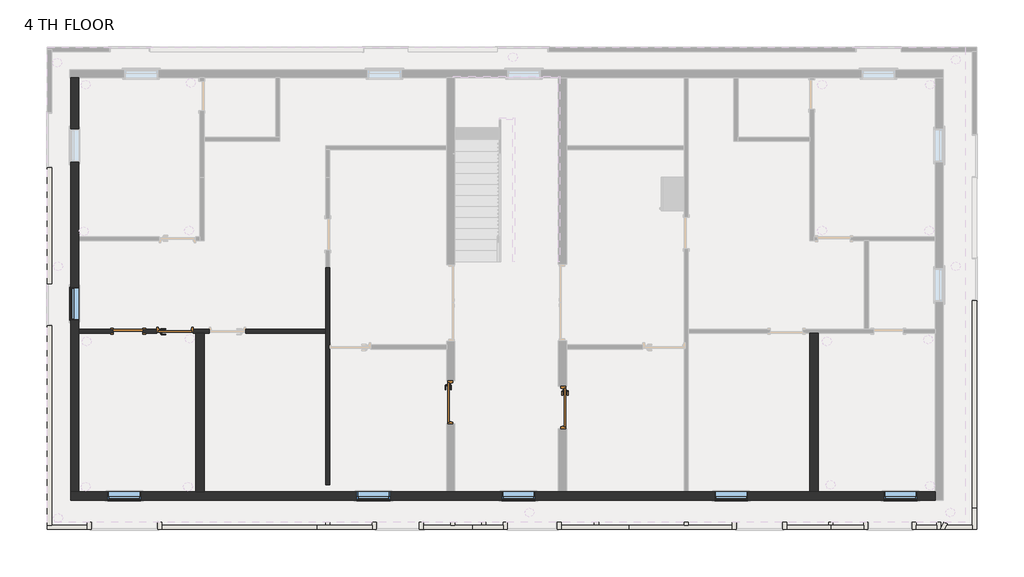
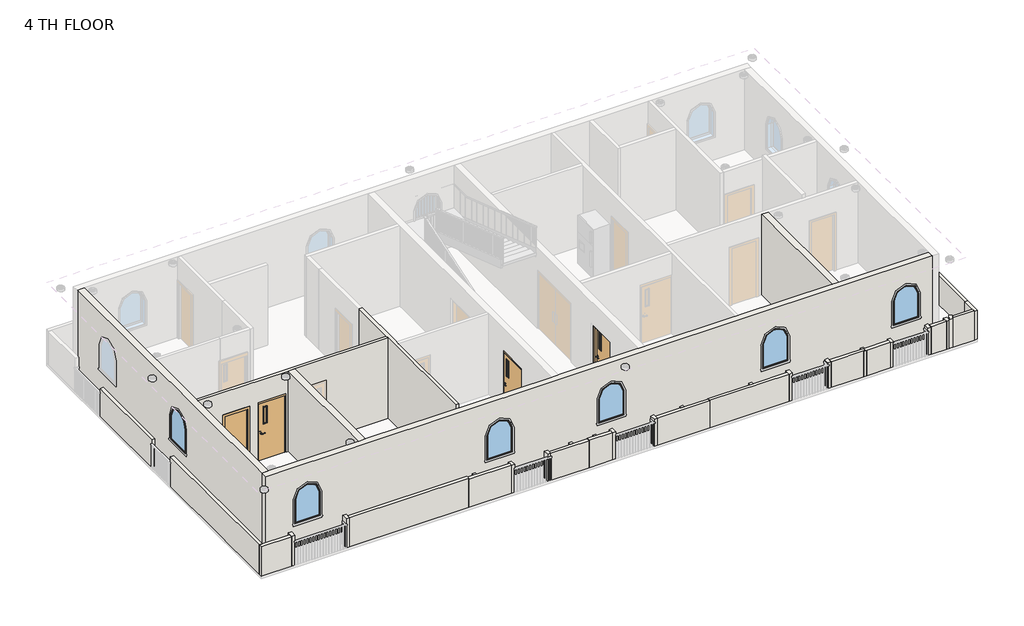
# One storey, part 1 of 7: 39 walls, 6 windows, 4 doors.
"""IFC4 building model written with IfcOpenShell, lengths in millimetres."""

from ifc_helpers import new_model, si_unit, frame, origin, place, context, project, spatial, polyline, circle_curve, outline, extrude, faceted_brep, transform, mapped, element, save
from ifc_brep_helpers import plane_surface, revolved_surface, advanced_brep
from components import door_586e558e, door_7d8f8091, door_passage_single_vision_lite_3_x7_38248cdf, door_d141acb4, window_fixed_round_top_3_x_4_dee2be1c

model = new_model("IFC4")

# Units and contexts
model_context = context("Model", 3, world=origin())
ifc_project = project(units=[si_unit("LENGTHUNIT", "METRE", prefix="MILLI")], contexts=[model_context])

# Site, building, storey
site = spatial("IfcSite", under=ifc_project)
building = spatial("IfcBuilding", under=site)
storey = spatial("IfcBuildingStorey", under=building, Name="4 TH FLOOR", Elevation=12801.6)

# Doors
placement = place(None, origin())
door_shape = door_586e558e(model_context)
element("IfcDoor", 1, ObjectType="Door-Passage-Single-Vision_Lite : 3'6\"X7' 2", at=placement, inside=storey, context=model_context, shape_type="MappedRepresentation", body=[
    mapped(door_shape, transform((1116.1432011, -1461.3932193, 12801.6), x_axis=(0.0, -1.0, 0.0), y_axis=(1.0, 0.0, 0.0), z_axis=(0.0, 0.0, 1.0))),
])
door_2_shape = door_7d8f8091(model_context)
element("IfcDoor", 2, ObjectType="Door-Passage-Single-Vision_Lite : 3'7\"X7' 3", at=placement, inside=storey, context=model_context, shape_type="MappedRepresentation", body=[
    mapped(door_2_shape, transform((-1956.7487998, -1318.7421379, 12801.6), x_axis=(0.0, -1.0, 0.0), y_axis=(1.0, 0.0, 0.0), z_axis=(0.0, 0.0, 1.0))),
])
door_passage_single_vision_lite_3_x7_shape = door_passage_single_vision_lite_3_x7_38248cdf(model_context)
element("IfcDoor", 3, ObjectType="Door-Passage-Single-Vision_Lite : 3'X7'", at=placement, inside=storey, context=model_context, shape_type="MappedRepresentation", body=[
    mapped(door_passage_single_vision_lite_3_x7_shape, transform((-9570.3987992, 646.8067334, 12801.6), x_axis=(1.0, 0.0, 0.0), y_axis=(0.0, 1.0, 0.0), z_axis=(0.0, 0.0, 1.0))),
])
door_3_shape = door_d141acb4(model_context)
element("IfcDoor", 4, ObjectType="Single-Flush : 2'8\"x 7'", at=placement, inside=storey, context=model_context, shape_type="MappedRepresentation", body=[
    mapped(door_3_shape, transform((-10865.7987992, 640.4567334, 12801.6), x_axis=(1.0, 0.0, 0.0), y_axis=(0.0, 1.0, 0.0), z_axis=(0.0, 0.0, 1.0))),
])

# Walls
element("IfcWall", 5, ObjectType="Generic - 4.5\"", at=placement, inside=storey, context=model_context, shape_type="Brep", body=[
    faceted_brep([(-10459.3987992, 583.3067334, 14935.2), (-10459.3987992, 583.3067334, 12801.6), (-10078.3987992, 583.3067334, 12801.6), (-10078.3987992, 583.3067334, 15036.8), (-9062.3987992, 583.3067334, 15036.8), (-9062.3987992, 583.3067334, 12801.6), (-8998.8987992, 583.3067334, 12801.6), (-8770.2987992, 583.3067334, 12801.6), (-8630.5987992, 583.3067334, 12801.6), (-8630.5987992, 583.3067334, 15036.8), (-7614.5987992, 583.3067334, 15036.8), (-7614.5987992, 583.3067334, 12801.6), (-5417.4987995, 583.3067334, 12801.6), (-5417.4987995, 583.3067334, 15849.6), (-8770.2987992, 583.3067334, 15849.6), (-8998.8987992, 583.3067334, 15849.6), (-12224.6987925, 583.3067334, 15849.6), (-12224.6987925, 583.3067334, 12801.6), (-11272.1987992, 583.3067334, 12801.6), (-11272.1987992, 583.3067334, 14935.2), (-10078.3987992, 697.6067334, 12801.6), (-10459.3987992, 697.6067334, 12801.6), (-10459.3987992, 697.6067334, 14935.2), (-11272.1987992, 697.6067334, 14935.2), (-11272.1987992, 697.6067334, 12801.6), (-12224.6987925, 697.6067334, 12801.6), (-12224.6987925, 697.6067334, 15849.6), (-5417.4987995, 697.6067334, 15849.6), (-5417.4987995, 697.6067334, 12801.6), (-7614.5987992, 697.6067334, 12801.6), (-7614.5987992, 697.6067334, 15036.8), (-8630.5987992, 697.6067334, 15036.8), (-8630.5987992, 697.6067334, 12801.6), (-9062.3987992, 697.6067334, 12801.6), (-9062.3987992, 697.6067334, 15036.8), (-10078.3987992, 697.6067334, 15036.8)], [[[0, 1, 2, 3, 4, 5, 6, 7, 8, 9, 10, 11, 12, 13, 14, 15, 16, 17, 18, 19]], [[20, 21, 22, 23, 24, 25, 26, 27, 28, 29, 30, 31, 32, 33, 34, 35]], [[28, 12, 11, 29]], [[32, 8, 7, 6, 5, 33]], [[18, 17, 25, 24]], [[2, 1, 21, 20]], [[16, 15, 14, 13, 27, 26]], [[17, 16, 26, 25]], [[13, 12, 28, 27]], [[9, 8, 32, 31]], [[10, 9, 31, 30]], [[11, 10, 30, 29]], [[4, 34, 33, 5]], [[34, 4, 3, 35]], [[35, 3, 2, 20]], [[22, 21, 1, 0]], [[23, 22, 0, 19]], [[24, 23, 19, 18]]]),
])
element("IfcWall", 6, ObjectType="Generic - 4.5\"", at=placement, inside=storey, context=model_context, shape_type="Brep", body=[
    faceted_brep([(-5417.4987995, 2399.4067802, 12801.6), (-5417.4987995, 697.6067334, 12801.6), (-5417.4987995, 583.3067334, 12801.6), (-5417.4987995, -3594.9932193, 12801.6), (-5417.4987995, -3594.9932193, 15849.6), (-5417.4987995, 583.3067334, 15849.6), (-5417.4987995, 697.6067334, 15849.6), (-5417.4987995, 2399.4067802, 15849.6), (-5303.1987995, -3594.9932193, 15849.6), (-5303.1987995, -3594.9932193, 12801.6), (-5303.1987995, 148.1078621, 12801.6), (-5303.1987995, 148.1078621, 15036.8), (-5303.1987995, 262.4078621, 15036.8), (-5303.1987995, 262.4078621, 12801.6), (-5303.1987995, 2399.4067802, 12801.6), (-5303.1987995, 2399.4067802, 15849.6), (-5303.1987995, 262.4078621, 15849.6), (-5303.1987995, 148.1078621, 15849.6), (-5334.9487995, 262.4078621, 12801.6), (-5334.9487995, 148.1078621, 12801.6), (-5334.9487995, 262.4078621, 15036.8), (-5334.9487995, 148.1078621, 15036.8)], [[[0, 1, 2, 3, 4, 5, 6, 7]], [[8, 9, 10, 11, 12, 13, 14, 15, 16, 17]], [[3, 2, 1, 0, 14, 13, 18, 19, 10, 9]], [[4, 3, 9, 8]], [[7, 6, 5, 4, 8, 17, 16, 15]], [[0, 7, 15, 14]], [[20, 18, 13, 12]], [[19, 21, 11, 10]], [[21, 20, 12, 11]], [[18, 20, 21, 19]]]),
])
element("IfcWall", 7, ObjectType="Generic - 4.5\"", at=placement, inside=storey, context=model_context, shape_type="Brep", body=[
    faceted_brep([(-13088.8067989, -4826.8932661, 12801.6), (-11996.6067989, -4826.8932661, 12801.6), (-11996.6067989, -4826.8932661, 13914.5417562), (-13088.8067989, -4826.8932661, 13914.5417562), (-13088.8067989, -4712.5932661, 12801.6), (-13088.8067989, -4712.5932661, 13914.5417562), (-11996.6067989, -4712.5932661, 13914.5417562), (-11996.6067989, -4712.5932661, 12801.6), (-12974.5067989, -4712.5932661, 12801.6)], [[[0, 1, 2, 3]], [[4, 5, 6, 7, 8]], [[1, 0, 4, 8, 7]], [[3, 2, 6, 5]], [[2, 1, 7, 6]], [[0, 3, 5, 4]]]),
])
element("IfcWall", 8, ObjectType="Generic - 4.5\"", at=placement, inside=storey, context=model_context, shape_type="Brep", body=[
    faceted_brep([(-11996.6067989, -4623.6932193, 12801.6), (-11996.6067989, -4712.5932661, 12801.6), (-11996.6067989, -4826.8932661, 12801.6), (-11996.6067989, -4826.8932661, 13914.5417562), (-11996.6067989, -4826.8932661, 13935.5303619), (-11996.6067989, -4623.6932193, 13935.5303619), (-11882.3067989, -4623.6932193, 12801.6), (-11882.3067989, -4623.6932193, 13935.5303619), (-11882.3067989, -4826.8932661, 13935.5303619), (-11882.3067989, -4826.8932661, 12801.6)], [[[0, 1, 2, 3, 4, 5]], [[6, 7, 8, 9]], [[2, 1, 0, 6, 9]], [[5, 4, 8, 7]], [[0, 5, 7, 6]], [[4, 3, 2, 9, 8]]]),
])
element("IfcWall", 9, ObjectType="Generic - 4.5\"", at=placement, inside=storey, context=model_context, shape_type="Brep", body=[
    faceted_brep([(11660.3143245, -4826.8932661, 12801.6), (12426.0012043, -4826.8932661, 12801.6), (12426.0012043, -4826.8932661, 13893.4617784), (12426.0012043, -4826.8932661, 13904.7196614), (11660.3143245, -4826.8932661, 13904.7196614), (11660.3143245, -4826.8932661, 13891.1342527), (11716.0621594, -4712.5932661, 12801.6), (11716.0621594, -4712.5932661, 13904.7196614), (12426.0012043, -4712.5932661, 13904.7196614), (12426.0012043, -4712.5932661, 12801.6)], [[[0, 1, 2, 3, 4, 5]], [[6, 7, 8, 9]], [[1, 0, 6, 9]], [[4, 3, 8, 7]], [[3, 2, 1, 9, 8]], [[0, 5, 4, 7, 6]]]),
])
element("IfcWall", 10, ObjectType="Generic - 4.5\"", at=placement, inside=storey, context=model_context, shape_type="Brep", body=[
    faceted_brep([(11632.2512075, -4623.6932193, 12801.6), (11533.1439227, -4826.8932661, 12801.6), (11533.1439227, -4826.8932661, 13891.1342527), (11632.2512075, -4623.6932193, 13891.1342527), (11734.983367, -4673.7990414, 12801.6), (11734.983367, -4673.7990414, 13891.1342527), (11660.3143245, -4826.8932661, 13891.1342527), (11660.3143245, -4826.8932661, 12801.6), (11716.0621594, -4712.5932661, 12801.6)], [[[0, 1, 2, 3]], [[4, 5, 6, 7, 8]], [[1, 0, 4, 8, 7]], [[3, 2, 6, 5]], [[0, 3, 5, 4]], [[2, 1, 7, 6]]]),
])
element("IfcWall", 11, ObjectType="Generic - 4.5\"", at=placement, inside=storey, context=model_context, shape_type="Brep", body=[
    faceted_brep([(12426.0012043, -4236.3432661, 12801.6), (12426.0012043, -4712.5932661, 12801.6), (12426.0012043, -4826.8932661, 12801.6), (12426.0012043, -4826.8932661, 13893.4617784), (12426.0012043, -4236.3432661, 13893.4617784), (12426.0012043, -4236.3432661, 13888.2712164), (12540.3012043, -4236.3432661, 12801.6), (12540.3012043, -4236.3432661, 13888.2712164), (12540.3012043, -4236.3432661, 13893.4617784), (12540.3012043, -4826.8932661, 13893.4617784), (12540.3012043, -4826.8932661, 12801.6)], [[[0, 1, 2, 3, 4, 5]], [[6, 7, 8, 9, 10]], [[2, 1, 0, 6, 10]], [[4, 3, 9, 8]], [[0, 5, 4, 8, 7, 6]], [[3, 2, 10, 9]]]),
])
element("IfcWall", 12, ObjectType="Generic - 4.5\"", at=placement, inside=storey, context=model_context, shape_type="SweptSolid", body=[
    extrude(outline(polyline([(-5417.4987995, -4712.5932661), (-5417.4987995, -4623.6932193), (-5303.1987995, -4623.6932193), (-5303.1987995, -4712.5932661), (-5417.4987995, -4712.5932661)])), frame((0.0, 0.0, 12801.6), z_axis=(0.0, 0.0, 1.0), x_axis=(1.0, 0.0, 0.0)), (0.0, 0.0, 1.0), 1063.0786215),
])
element("IfcWall", 13, ObjectType="Generic - 4.5\"", at=placement, inside=storey, context=model_context, shape_type="Brep", body=[
    faceted_brep([(-5663.8033402, -4826.8932661, 12801.6), (-4134.7987995, -4826.8932661, 12801.6), (-4134.7987995, -4826.8932661, 13860.7218247), (-4134.7987995, -4826.8932661, 13868.8575049), (-5663.8033402, -4826.8932661, 13868.8575049), (-5663.8033402, -4712.5932661, 12801.6), (-5663.8033402, -4712.5932661, 13868.8575049), (-4134.7987995, -4712.5932661, 13868.8575049), (-4134.7987995, -4712.5932661, 12801.6), (-5303.1987995, -4712.5932661, 12801.6), (-5417.4987995, -4712.5932661, 12801.6)], [[[0, 1, 2, 3, 4]], [[5, 6, 7, 8, 9, 10]], [[1, 0, 5, 10, 9, 8]], [[4, 3, 7, 6]], [[0, 4, 6, 5]], [[3, 2, 1, 8, 7]]]),
])
element("IfcWall", 14, ObjectType="Generic - 4.5\"", at=placement, inside=storey, context=model_context, shape_type="Brep", body=[
    faceted_brep([(-2725.0987995, -4826.8932661, 12801.6), (-1354.4417672, -4826.8932661, 12801.6), (-1354.4417672, -4826.8932661, 13817.6), (-2725.0987995, -4826.8932661, 13817.6), (-2725.0987995, -4712.5932661, 12801.6), (-2725.0987995, -4712.5932661, 13817.6), (-1354.4417672, -4712.5932661, 13817.6), (-1354.4417672, -4712.5932661, 12801.6), (-1848.7987998, -4712.5932661, 12801.6), (-1963.0987998, -4712.5932661, 12801.6)], [[[0, 1, 2, 3]], [[4, 5, 6, 7, 8, 9]], [[1, 0, 4, 9, 8, 7]], [[2, 1, 7, 6]], [[3, 2, 6, 5]], [[0, 3, 5, 4]]]),
])
element("IfcWall", 15, ObjectType="Generic - 4.5\"", at=placement, inside=storey, context=model_context, shape_type="SweptSolid", body=[
    extrude(outline(polyline([(-1963.0987998, -4712.5932661), (-1963.0987998, -4623.6932193), (-1848.7987998, -4623.6932193), (-1848.7987998, -4712.5932661), (-1963.0987998, -4712.5932661)])), frame((0.0, 0.0, 12801.6), z_axis=(0.0, 0.0, 1.0), x_axis=(1.0, 0.0, 0.0)), (0.0, 0.0, 1.0), 1029.3234006),
])
element("IfcWall", 16, ObjectType="Generic - 4.5\"", at=placement, inside=storey, context=model_context, shape_type="SweptSolid", body=[
    extrude(outline(polyline([(-1112.1987998, -4712.5932661), (-1112.1987998, -4623.6932193), (-997.8987998, -4623.6932193), (-997.8987998, -4712.5932661), (-1112.1987998, -4712.5932661)])), frame((0.0, 0.0, 12801.6), z_axis=(0.0, 0.0, 1.0), x_axis=(1.0, 0.0, 0.0)), (0.0, 0.0, 1.0), 1016.0),
])
element("IfcWall", 17, ObjectType="Generic - 4.5\"", at=placement, inside=storey, context=model_context, shape_type="SweptSolid", body=[
    extrude(outline(polyline([(1999.3012002, -4712.5932661), (1999.3012002, -4623.6932193), (2113.6012002, -4623.6932193), (2113.6012002, -4712.5932661), (1999.3012002, -4712.5932661)])), frame((0.0, 0.0, 12801.6), z_axis=(0.0, 0.0, 1.0), x_axis=(1.0, 0.0, 0.0)), (0.0, 0.0, 1.0), 1013.2250283),
])
element("IfcWall", 18, ObjectType="Generic - 4.5\"", at=placement, inside=storey, context=model_context, shape_type="SweptSolid", body=[
    extrude(outline(polyline([(4475.8012082, -4712.5932661), (4475.8012082, -4623.6932193), (4590.1012082, -4623.6932193), (4590.1012082, -4712.5932661), (4475.8012082, -4712.5932661)])), frame((0.0, 0.0, 12801.6), z_axis=(0.0, 0.0, 1.0), x_axis=(1.0, 0.0, 0.0)), (0.0, 0.0, 1.0), 1027.4591445),
])
element("IfcWall", 19, ObjectType="Generic - 4.5\"", at=placement, inside=storey, context=model_context, shape_type="Brep", body=[
    faceted_brep([(2962.6087812, -4826.8932661, 12801.6), (5802.9512082, -4826.8932661, 12801.6), (5802.9512082, -4826.8932661, 13829.0591445), (2962.6087812, -4826.8932661, 13829.0591445), (2962.6087812, -4826.8932661, 13814.8250283), (2962.6087812, -4712.5932661, 12801.6), (2962.6087812, -4712.5932661, 13814.8250283), (2962.6087812, -4712.5932661, 13829.0591445), (4475.8012082, -4712.5932661, 13829.0591445), (4590.1012082, -4712.5932661, 13829.0591445), (5802.9512082, -4712.5932661, 13829.0591445), (5802.9512082, -4712.5932661, 12801.6), (4590.1012082, -4712.5932661, 12801.6), (4475.8012082, -4712.5932661, 12801.6)], [[[0, 1, 2, 3, 4]], [[5, 6, 7, 8, 9, 10, 11, 12, 13]], [[1, 0, 5, 13, 12, 11]], [[3, 2, 10, 9, 8, 7]], [[0, 4, 3, 7, 6, 5]], [[2, 1, 11, 10]]]),
])
element("IfcWall", 20, ObjectType="Generic - 4.5\"", at=placement, inside=storey, context=model_context, shape_type="Brep", body=[
    faceted_brep([(5802.9512082, -4623.6932193, 12801.6), (5802.9512082, -4712.5932661, 12801.6), (5802.9512082, -4826.8932661, 12801.6), (5802.9512082, -4826.8932661, 13829.0591445), (5802.9512082, -4826.8932661, 13833.9822201), (5802.9512082, -4623.6932193, 13833.9822201), (5917.2512082, -4623.6932193, 12801.6), (5917.2512082, -4623.6932193, 13833.9822201), (5917.2512082, -4826.8932661, 13833.9822201), (5917.2512082, -4826.8932661, 12801.6)], [[[0, 1, 2, 3, 4, 5]], [[6, 7, 8, 9]], [[2, 1, 0, 6, 9]], [[5, 4, 8, 7]], [[0, 5, 7, 6]], [[4, 3, 2, 9, 8]]]),
])
element("IfcWall", 21, ObjectType="Generic - 4.5\"", at=placement, inside=storey, context=model_context, shape_type="Brep", body=[
    faceted_brep([(7190.3011643, -4623.6932193, 12801.6), (7190.3011643, -4826.8932661, 12801.6), (7190.3011643, -4826.8932661, 13774.4158009), (7190.3011643, -4623.6932193, 13774.4158009), (7304.6011643, -4623.6932193, 12801.6), (7304.6011643, -4623.6932193, 13774.4158009), (7304.6011643, -4712.5932661, 13774.4158009), (7304.6011643, -4826.8932661, 13774.4158009), (7304.6011643, -4826.8932661, 12801.6), (7304.6011643, -4712.5932661, 12801.6)], [[[0, 1, 2, 3]], [[4, 5, 6, 7, 8, 9]], [[1, 0, 4, 9, 8]], [[3, 2, 7, 6, 5]], [[0, 3, 5, 4]], [[2, 1, 8, 7]]]),
])
element("IfcWall", 22, ObjectType="Generic - 4.5\"", at=placement, inside=storey, context=model_context, shape_type="Brep", body=[
    faceted_brep([(7304.6011643, -4826.8932661, 12801.6), (8463.6012082, -4826.8932661, 12801.6), (8463.6012082, -4826.8932661, 13758.0159658), (8520.7512082, -4826.8932661, 13758.0159658), (8520.7512082, -4826.8932661, 13771.280309), (8520.7512082, -4826.8932661, 13774.5581334), (7304.6011643, -4826.8932661, 13774.5581334), (7304.6011643, -4712.5932661, 12801.6), (7304.6011643, -4712.5932661, 13774.5581334), (8520.7512082, -4712.5932661, 13774.5581334), (8520.7512082, -4712.5932661, 13771.280309), (8520.7512082, -4712.5932661, 13758.0159658), (8463.6012082, -4712.5932661, 13758.0159658), (8463.6012082, -4712.5932661, 12801.6)], [[[0, 1, 2, 3, 4, 5, 6]], [[7, 8, 9, 10, 11, 12, 13]], [[1, 0, 7, 13]], [[6, 5, 9, 8]], [[0, 6, 8, 7]], [[5, 4, 3, 11, 10, 9]], [[11, 3, 2, 12]], [[2, 1, 13, 12]]]),
])
element("IfcWall", 23, ObjectType="Generic - 4.5\"", at=placement, inside=storey, context=model_context, shape_type="Brep", body=[
    faceted_brep([(8463.6012082, -4623.6932193, 12801.6), (8463.6012082, -4712.5932661, 12801.6), (8463.6012082, -4826.8932661, 12801.6), (8463.6012082, -4826.8932661, 13758.0159658), (8463.6012082, -4712.5932661, 13758.0159658), (8463.6012082, -4623.6932193, 13758.0159658), (8577.9012082, -4623.6932193, 12801.6), (8577.9012082, -4623.6932193, 13758.0159658), (8577.9012082, -4712.5932661, 13758.0159658), (8577.9012082, -4826.8932661, 13758.0159658), (8577.9012082, -4826.8932661, 12801.6), (8577.9012082, -4712.5932661, 12801.6), (8520.7512082, -4826.8932661, 13758.0159658)], [[[0, 1, 2, 3, 4, 5]], [[6, 7, 8, 9, 10, 11]], [[2, 1, 0, 6, 11, 10]], [[5, 4, 3, 12, 9, 8, 7]], [[0, 5, 7, 6]], [[3, 2, 10, 9, 12]]]),
])
element("IfcWall", 24, ObjectType="Generic - 4.5\"", at=placement, inside=storey, context=model_context, shape_type="Brep", body=[
    faceted_brep([(8577.9012082, -4826.8932661, 12801.6), (9422.4512082, -4826.8932661, 12801.6), (9422.4512082, -4826.8932661, 13753.8060641), (9422.4512082, -4826.8932661, 13771.280309), (8520.7512082, -4826.8932661, 13771.280309), (8520.7512082, -4826.8932661, 13758.0159658), (8577.9012082, -4826.8932661, 13758.0159658), (8577.9012082, -4712.5932661, 12801.6), (8577.9012082, -4712.5932661, 13758.0159658), (8520.7512082, -4712.5932661, 13758.0159658), (8520.7512082, -4712.5932661, 13771.280309), (9422.4512082, -4712.5932661, 13771.280309), (9422.4512082, -4712.5932661, 12801.6)], [[[0, 1, 2, 3, 4, 5, 6]], [[7, 8, 9, 10, 11, 12]], [[1, 0, 7, 12]], [[4, 3, 11, 10]], [[3, 2, 1, 12, 11]], [[5, 4, 10, 9]], [[5, 9, 8, 6]], [[0, 6, 8, 7]]]),
])
element("IfcWall", 25, ObjectType="Generic - 4.5\"", at=placement, inside=storey, context=model_context, shape_type="Brep", body=[
    faceted_brep([(9422.4512082, -4623.6932193, 12801.6), (9422.4512082, -4712.5932661, 12801.6), (9422.4512082, -4826.8932661, 12801.6), (9422.4512082, -4826.8932661, 13753.8060641), (9422.4512082, -4623.6932193, 13753.8060641), (9536.7512082, -4623.6932193, 12801.6), (9536.7512082, -4623.6932193, 13753.8060641), (9536.7512082, -4826.8932661, 13753.8060641), (9536.7512082, -4826.8932661, 12801.6)], [[[0, 1, 2, 3, 4]], [[5, 6, 7, 8]], [[2, 1, 0, 5, 8]], [[4, 3, 7, 6]], [[0, 4, 6, 5]], [[3, 2, 8, 7]]]),
])
element("IfcWall", 26, ObjectType="Generic - 4.5\"", at=placement, inside=storey, context=model_context, shape_type="Brep", body=[
    faceted_brep([(10764.1617205, -4623.6932193, 12801.6), (10764.1617205, -4826.8932661, 12801.6), (10764.1617205, -4826.8932661, 13827.9072304), (10764.1617205, -4623.6932193, 13827.9072304), (10878.4617205, -4623.6932193, 12801.6), (10878.4617205, -4623.6932193, 13827.9072304), (10878.4617205, -4826.8932661, 13827.9072304), (10878.4617205, -4826.8932661, 12801.6), (10878.4617205, -4712.5932661, 12801.6)], [[[0, 1, 2, 3]], [[4, 5, 6, 7, 8]], [[1, 0, 4, 8, 7]], [[3, 2, 6, 5]], [[0, 3, 5, 4]], [[2, 1, 7, 6]]]),
])
element("IfcWall", 27, ObjectType="Generic - 4.5\"", at=placement, inside=storey, context=model_context, shape_type="Brep", body=[
    faceted_brep([(10878.4617205, -4826.8932661, 12801.6), (11437.2617205, -4826.8932661, 12801.6), (11437.2617205, -4826.8932661, 13850.2912221), (10878.4617205, -4826.8932661, 13850.2912221), (10878.4617205, -4826.8932661, 13827.9072304), (10878.4617205, -4712.5932661, 12801.6), (10878.4617205, -4712.5932661, 13850.2912221), (11437.2617205, -4712.5932661, 13850.2912221), (11437.2617205, -4712.5932661, 12801.6)], [[[0, 1, 2, 3, 4]], [[5, 6, 7, 8]], [[1, 0, 5, 8]], [[3, 2, 7, 6]], [[0, 4, 3, 6, 5]], [[2, 1, 8, 7]]]),
])
element("IfcWall", 28, ObjectType="Generic - 4.5\"", at=placement, inside=storey, context=model_context, shape_type="Brep", body=[
    faceted_brep([(11437.2617205, -4623.6932193, 12801.6), (11437.2617205, -4712.5932661, 12801.6), (11437.2617205, -4826.8932661, 12801.6), (11437.2617205, -4826.8932661, 13850.2912221), (11437.2617205, -4712.5932661, 13850.2912221), (11437.2617205, -4623.6932193, 13850.2912221), (11551.5617205, -4623.6932193, 12801.6), (11551.5617205, -4623.6932193, 13850.2912221), (11551.5617205, -4826.8932661, 13850.2912221), (11551.5617205, -4826.8932661, 12801.6)], [[[0, 1, 2, 3, 4, 5]], [[6, 7, 8, 9]], [[2, 1, 0, 6, 9]], [[5, 4, 3, 8, 7]], [[0, 5, 7, 6]], [[3, 2, 9, 8]]]),
])
element("IfcWall", 29, ObjectType="Generic - 4.5\"", at=placement, inside=storey, context=model_context, shape_type="Brep", body=[
    faceted_brep([(-4134.7987995, -4623.6932193, 12801.6), (-4134.7987995, -4712.5932661, 12801.6), (-4134.7987995, -4826.8932661, 12801.6), (-4134.7987995, -4826.8932661, 13860.7218247), (-4134.7987995, -4623.6932193, 13860.7218247), (-4020.4987995, -4623.6932193, 12801.6), (-4020.4987995, -4623.6932193, 13860.7218247), (-4020.4987995, -4826.8932661, 13860.7218247), (-4020.4987995, -4826.8932661, 12801.6)], [[[0, 1, 2, 3, 4]], [[5, 6, 7, 8]], [[2, 1, 0, 5, 8]], [[4, 3, 7, 6]], [[0, 4, 6, 5]], [[3, 2, 8, 7]]]),
])
element("IfcWall", 30, ObjectType="Generic - 4.5\"", at=placement, inside=storey, context=model_context, shape_type="Brep", body=[
    faceted_brep([(-2839.3987995, -4623.6932193, 12801.6), (-2839.3987995, -4826.8932661, 12801.6), (-2839.3987995, -4826.8932661, 13818.3549618), (-2839.3987995, -4623.6932193, 13818.3549618), (-2725.0987995, -4623.6932193, 12801.6), (-2725.0987995, -4623.6932193, 13818.3549618), (-2725.0987995, -4826.8932661, 13818.3549618), (-2725.0987995, -4826.8932661, 13817.6), (-2725.0987995, -4826.8932661, 12801.6), (-2725.0987995, -4712.5932661, 12801.6)], [[[0, 1, 2, 3]], [[4, 5, 6, 7, 8, 9]], [[1, 0, 4, 9, 8]], [[3, 2, 6, 5]], [[0, 3, 5, 4]], [[2, 1, 8, 7, 6]]]),
])
element("IfcWall", 31, ObjectType="Generic - 4.5\"", at=placement, inside=storey, context=model_context, shape_type="Brep", body=[
    faceted_brep([(-1354.4417672, -4826.8932661, 12801.6), (-520.5065315, -4826.8932661, 12801.6), (-520.5065315, -4826.8932661, 13825.4796817), (-520.5065315, -4826.8932661, 13832.740074), (-1354.4417672, -4826.8932661, 13832.740074), (-1354.4417672, -4826.8932661, 13817.6), (-1354.4417672, -4712.5932661, 12801.6), (-1354.4417672, -4712.5932661, 13817.6), (-1354.4417672, -4712.5932661, 13832.740074), (-520.5065315, -4712.5932661, 13832.740074), (-520.5065315, -4712.5932661, 12801.6), (-997.8987998, -4712.5932661, 12801.6), (-1112.1987998, -4712.5932661, 12801.6)], [[[0, 1, 2, 3, 4, 5]], [[6, 7, 8, 9, 10, 11, 12]], [[1, 0, 6, 12, 11, 10]], [[4, 3, 9, 8]], [[0, 5, 4, 8, 7, 6]], [[3, 2, 1, 10, 9]]]),
])
element("IfcWall", 32, ObjectType="Generic - 4.5\"", at=placement, inside=storey, context=model_context, shape_type="Brep", body=[
    faceted_brep([(-520.5065315, -4623.6932193, 12801.6), (-520.5065315, -4712.5932661, 12801.6), (-520.5065315, -4826.8932661, 12801.6), (-520.5065315, -4826.8932661, 13825.4796817), (-520.5065315, -4623.6932193, 13825.4796817), (-406.2065315, -4623.6932193, 12801.6), (-406.2065315, -4623.6932193, 13825.4796817), (-406.2065315, -4826.8932661, 13825.4796817), (-406.2065315, -4826.8932661, 12801.6)], [[[0, 1, 2, 3, 4]], [[5, 6, 7, 8]], [[2, 1, 0, 5, 8]], [[4, 3, 7, 6]], [[0, 4, 6, 5]], [[3, 2, 8, 7]]]),
])
element("IfcWall", 33, ObjectType="Generic - 4.5\"", at=placement, inside=storey, context=model_context, shape_type="Brep", body=[
    faceted_brep([(970.0932011, -4623.6932193, 12801.6), (970.0932011, -4826.8932661, 12801.6), (970.0932011, -4826.8932661, 13814.8250283), (970.0932011, -4623.6932193, 13814.8250283), (1084.3932011, -4623.6932193, 12801.6), (1084.3932011, -4623.6932193, 13814.8250283), (1084.3932011, -4712.5932661, 13814.8250283), (1084.3932011, -4826.8932661, 13814.8250283), (1084.3932011, -4826.8932661, 12801.6), (1084.3932011, -4712.5932661, 12801.6)], [[[0, 1, 2, 3]], [[4, 5, 6, 7, 8, 9]], [[1, 0, 4, 9, 8]], [[3, 2, 7, 6, 5]], [[0, 3, 5, 4]], [[2, 1, 8, 7]]]),
])
element("IfcWall", 34, ObjectType="Generic - 4.5\"", at=placement, inside=storey, context=model_context, shape_type="Brep", body=[
    faceted_brep([(1084.3932011, -4826.8932661, 12801.6), (2962.6087812, -4826.8932661, 12801.6), (2962.6087812, -4826.8932661, 13814.8250283), (1084.3932011, -4826.8932661, 13814.8250283), (1084.3932011, -4712.5932661, 12801.6), (1084.3932011, -4712.5932661, 13814.8250283), (1999.3012002, -4712.5932661, 13814.8250283), (2113.6012002, -4712.5932661, 13814.8250283), (2962.6087812, -4712.5932661, 13814.8250283), (2962.6087812, -4712.5932661, 12801.6), (2113.6012002, -4712.5932661, 12801.6), (1999.3012002, -4712.5932661, 12801.6)], [[[0, 1, 2, 3]], [[4, 5, 6, 7, 8, 9, 10, 11]], [[1, 0, 4, 11, 10, 9]], [[2, 1, 9, 8]], [[3, 2, 8, 7, 6, 5]], [[0, 3, 5, 4]]]),
])
element("IfcWall", 35, ObjectType="Generic - 4.5\"", at=placement, inside=storey, context=model_context, shape_type="Brep", body=[
    faceted_brep([(-10045.9470335, -4623.6932193, 12801.6), (-10045.9470335, -4826.8932661, 12801.6), (-10045.9470335, -4826.8932661, 13909.304535), (-10045.9470335, -4623.6932193, 13909.304535), (-9931.6470335, -4623.6932193, 12801.6), (-9931.6470335, -4623.6932193, 13909.304535), (-9931.6470335, -4712.5932661, 13909.304535), (-9931.6470335, -4826.8932661, 13909.304535), (-9931.6470335, -4826.8932661, 12801.6), (-9931.6470335, -4712.5932661, 12801.6)], [[[0, 1, 2, 3]], [[4, 5, 6, 7, 8, 9]], [[1, 0, 4, 9, 8]], [[3, 2, 7, 6, 5]], [[0, 3, 5, 4]], [[2, 1, 8, 7]]]),
])
element("IfcWall", 36, ObjectType="Generic - 4.5\"", at=placement, inside=storey, context=model_context, shape_type="Brep", body=[
    faceted_brep([(-9931.6470335, -4826.8932661, 12801.6), (-5663.8033402, -4826.8932661, 12801.6), (-5663.8033402, -4826.8932661, 13868.8575049), (-5663.8033402, -4826.8932661, 13909.304535), (-9931.6470335, -4826.8932661, 13909.304535), (-9931.6470335, -4712.5932661, 12801.6), (-9931.6470335, -4712.5932661, 13909.304535), (-5663.8033402, -4712.5932661, 13909.304535), (-5663.8033402, -4712.5932661, 13868.8575049), (-5663.8033402, -4712.5932661, 12801.6)], [[[0, 1, 2, 3, 4]], [[5, 6, 7, 8, 9]], [[1, 0, 5, 9]], [[3, 2, 1, 9, 8, 7]], [[4, 3, 7, 6]], [[0, 4, 6, 5]]]),
])
element("IfcWall", 37, ObjectType="Generic - 4.5\"", at=placement, inside=storey, context=model_context, shape_type="Brep", body=[
    faceted_brep([(-13088.8067989, 792.8567339, 12801.6), (-13088.8067989, -4712.5932661, 12801.6), (-13088.8067989, -4712.5932661, 13914.5417562), (-13088.8067989, -4712.5932661, 13915.767936), (-13088.8067989, 792.8567339, 13915.767936), (-12974.5067989, 792.8567339, 12801.6), (-12974.5067989, 792.8567339, 13915.767936), (-12974.5067989, -4712.5932661, 13915.767936), (-12974.5067989, -4712.5932661, 12801.6)], [[[0, 1, 2, 3, 4]], [[5, 6, 7, 8]], [[1, 0, 5, 8]], [[4, 3, 7, 6]], [[0, 4, 6, 5]], [[3, 2, 1, 8, 7]]]),
])
element("IfcWall", 38, ObjectType="Generic - 4.5\"", at=placement, inside=storey, context=model_context, shape_type="SweptSolid", body=[
    extrude(outline(polyline([(-12976.0338648, 5154.3604213), (-12976.0338648, 1953.9604213), (-13090.3338648, 1953.9604213), (-13090.3338648, 5154.3604213), (-12976.0338648, 5154.3604213)])), frame((0.0, 0.0, 12801.6), z_axis=(0.0, 0.0, 1.0), x_axis=(1.0, 0.0, 0.0)), (0.0, 0.0, 1.0), 1047.4413329),
])
element("IfcWall", 39, ObjectType="Generic - 4.5\"", at=placement, inside=storey, context=model_context, shape_type="SweptSolid", body=[
    extrude(outline(polyline([(12426.0012043, -4236.3432661), (12426.0012043, 1478.6567334), (12540.3012043, 1478.6567334), (12540.3012043, -4236.3432661), (12426.0012043, -4236.3432661)])), frame((0.0, 0.0, 12801.6), z_axis=(0.0, 0.0, 1.0), x_axis=(1.0, 0.0, 0.0)), (0.0, 0.0, 1.0), 1086.6712164),
])
element("IfcWall", 40, ObjectType="Generic - 9\"", at=placement, inside=storey, context=model_context, shape_type="AdvancedBrep", body=[
    advanced_brep(
    [(11397.3012075, -3785.4932193, 12801.6), (8171.5012079, -3785.4932193, 12801.6), (7942.9012079, -3785.4932193, 12801.6), (4590.1012082, -3785.4932193, 12801.6), (4475.8012082, -3785.4932193, 12801.6), (1236.7932011, -3785.4932193, 12801.6), (1008.1932011, -3785.4932193, 12801.6), (-1848.7987998, -3785.4932193, 12801.6), (-2077.3987998, -3785.4932193, 12801.6), (-8770.2987992, -3785.4932193, 12801.6), (-8998.8987992, -3785.4932193, 12801.6), (-12224.6987925, -3785.4932193, 12801.6), (-12453.2987925, -3785.4932193, 12801.6), (-12453.2987925, -3785.4932193, 15849.6), (-12224.6987925, -3785.4932193, 15849.6), (-8998.8987992, -3785.4932193, 15849.6), (-8770.2987992, -3785.4932193, 15849.6), (-2077.3987998, -3785.4932193, 15849.6), (-1848.7987998, -3785.4932193, 15849.6), (1008.1932011, -3785.4932193, 15849.6), (1236.7932011, -3785.4932193, 15849.6), (4475.8012082, -3785.4932193, 15849.6), (4590.1012082, -3785.4932193, 15849.6), (7942.9012079, -3785.4932193, 15849.6), (8171.5012079, -3785.4932193, 15849.6), (11397.3012075, -3785.4932193, 15849.6), (-10510.1987925, -3785.4932193, 13716.0), (-10510.1987925, -3785.4932193, 14630.4), (-11424.5987925, -3785.4932193, 14630.4), (-11424.5987925, -3785.4932193, 13716.0), (-3639.4987998, -3785.4932193, 13716.0), (-3639.4987998, -3785.4932193, 14630.4), (-4553.8987998, -3785.4932193, 14630.4), (-4553.8987998, -3785.4932193, 13716.0), (360.4932011, -3785.4932193, 13716.0), (360.4932011, -3785.4932193, 14630.4), (-553.9067989, -3785.4932193, 14630.4), (-553.9067989, -3785.4932193, 13716.0), (6228.4012079, -3785.4932193, 13716.0), (6228.4012079, -3785.4932193, 14630.4), (5314.0012079, -3785.4932193, 14630.4), (5314.0012079, -3785.4932193, 13716.0), (10902.0012075, -3785.4932193, 13716.0), (10902.0012075, -3785.4932193, 14630.4), (9987.6012075, -3785.4932193, 14630.4), (9987.6012075, -3785.4932193, 13716.0), (11397.3012075, -4014.0932193, 12801.6), (11397.3012075, -4014.0932193, 15849.6), (-12453.2987925, -4014.0932193, 15849.6), (-12453.2987925, -4014.0932193, 12801.6), (-10510.1987925, -4014.0932193, 13716.0), (-11424.5987925, -4014.0932193, 13716.0), (-11424.5987925, -4014.0932193, 14630.4), (-10510.1987925, -4014.0932193, 14630.4), (-3639.4987998, -4014.0932193, 13716.0), (-4553.8987998, -4014.0932193, 13716.0), (-4553.8987998, -4014.0932193, 14630.4), (-3639.4987998, -4014.0932193, 14630.4), (360.4932011, -4014.0932193, 13716.0), (-553.9067989, -4014.0932193, 13716.0), (-553.9067989, -4014.0932193, 14630.4), (360.4932011, -4014.0932193, 14630.4), (6228.4012079, -4014.0932193, 13716.0), (5314.0012079, -4014.0932193, 13716.0), (5314.0012079, -4014.0932193, 14630.4), (6228.4012079, -4014.0932193, 14630.4), (10902.0012075, -4014.0932193, 13716.0), (9987.6012075, -4014.0932193, 13716.0), (9987.6012075, -4014.0932193, 14630.4), (10902.0012075, -4014.0932193, 14630.4)],
    [
        (0, 1),
        (1, 2),
        (2, 3),
        (3, 4),
        (4, 5),
        (5, 6),
        (6, 7),
        (7, 8),
        (8, 9),
        (9, 10),
        (10, 11),
        (11, 12),
        (12, 13),
        (13, 14),
        (14, 15),
        (15, 16),
        (16, 17),
        (17, 18),
        (18, 19),
        (19, 20),
        (20, 21),
        (21, 22),
        (22, 23),
        (23, 24),
        (24, 25),
        (25, 0),
        (26, 27),
        (27, 28, circle_curve(frame((-10967.3987925, -3785.4932193, 14630.4), z_axis=(0.0, -1.0, 0.0), x_axis=(-1.0, 0.0, 0.0)), 457.2)),
        (28, 29),
        (29, 26),
        (30, 31),
        (31, 32, circle_curve(frame((-4096.6987998, -3785.4932193, 14630.4), z_axis=(0.0, -1.0, 0.0), x_axis=(-1.0, 0.0, 0.0)), 457.2)),
        (32, 33),
        (33, 30),
        (34, 35),
        (35, 36, circle_curve(frame((-96.7067989, -3785.4932193, 14630.4), z_axis=(0.0, -1.0, 0.0), x_axis=(-1.0, 0.0, 0.0)), 457.2)),
        (36, 37),
        (37, 34),
        (38, 39),
        (39, 40, circle_curve(frame((5771.2012079, -3785.4932193, 14630.4), z_axis=(0.0, -1.0, 0.0), x_axis=(-1.0, 0.0, 0.0)), 457.2)),
        (40, 41),
        (41, 38),
        (42, 43),
        (43, 44, circle_curve(frame((10444.8012075, -3785.4932193, 14630.4), z_axis=(0.0, -1.0, 0.0), x_axis=(-1.0, 0.0, 0.0)), 457.2)),
        (44, 45),
        (45, 42),
        (46, 47),
        (47, 48),
        (48, 49),
        (49, 46),
        (50, 51),
        (51, 52),
        (52, 53, circle_curve(frame((-10967.3987925, -4014.0932193, 14630.4), z_axis=(0.0, 1.0, 0.0), x_axis=(-1.0, 0.0, 0.0)), 457.2)),
        (53, 50),
        (54, 55),
        (55, 56),
        (56, 57, circle_curve(frame((-4096.6987998, -4014.0932193, 14630.4), z_axis=(0.0, 1.0, 0.0), x_axis=(-1.0, 0.0, 0.0)), 457.2)),
        (57, 54),
        (58, 59),
        (59, 60),
        (60, 61, circle_curve(frame((-96.7067989, -4014.0932193, 14630.4), z_axis=(0.0, 1.0, 0.0), x_axis=(-1.0, 0.0, 0.0)), 457.2)),
        (61, 58),
        (62, 63),
        (63, 64),
        (64, 65, circle_curve(frame((5771.2012079, -4014.0932193, 14630.4), z_axis=(0.0, 1.0, 0.0), x_axis=(-1.0, 0.0, 0.0)), 457.2)),
        (65, 62),
        (66, 67),
        (67, 68),
        (68, 69, circle_curve(frame((10444.8012075, -4014.0932193, 14630.4), z_axis=(0.0, 1.0, 0.0), x_axis=(-1.0, 0.0, 0.0)), 457.2)),
        (69, 66),
        (0, 46),
        (49, 12),
        (13, 48),
        (47, 25),
        (50, 26),
        (29, 51),
        (28, 52),
        (27, 53),
        (54, 30),
        (33, 55),
        (32, 56),
        (31, 57),
        (58, 34),
        (37, 59),
        (36, 60),
        (35, 61),
        (62, 38),
        (41, 63),
        (40, 64),
        (39, 65),
        (66, 42),
        (45, 67),
        (44, 68),
        (43, 69),
    ],
    [
        plane_surface(frame((11386.6090247, -3785.4932193, 12801.6), z_axis=(0.0, 1.0, 0.0), x_axis=(-1.0, 0.0, 0.0))),
        plane_surface(frame((11386.6090247, -4014.0932193, 12801.6), z_axis=(0.0, -1.0, 0.0), x_axis=(1.0, 0.0, 0.0))),
        plane_surface(frame((11511.6012075, -3785.4932193, 12801.6), z_axis=(0.0, 0.0, -1.0), x_axis=(0.0, -1.0, 0.0))),
        plane_surface(frame((-12338.9987925, -3785.4932193, 15849.6), z_axis=(0.0, 0.0, 1.0), x_axis=(0.0, -1.0, 0.0))),
        plane_surface(frame((11397.3012075, 7629.6366753, 12801.6), z_axis=(1.0, 0.0, 0.0), x_axis=(0.0, -1.0, 0.0))),
        plane_surface(frame((-12453.2987925, -3782.6829884, 12801.6), z_axis=(-1.0, 0.0, 0.0), x_axis=(0.0, -1.0, 0.0))),
        plane_surface(frame((-10510.1987925, -4014.0932193, 13716.0), z_axis=(0.0, 0.0, 1.0), x_axis=(0.0, 1.0, 0.0))),
        plane_surface(frame((-11424.5987925, -4014.0932193, 13716.0), z_axis=(1.0, 0.0, 0.0), x_axis=(0.0, 1.0, 0.0))),
        revolved_surface(polyline([(-11424.5987925, -3785.4932193, 14630.4), (-11424.5987925, -4014.0932193, 14630.4)]), (-10967.3987925, -3785.4932193, 14630.4), (0.0, 1.0, 0.0)),
        plane_surface(frame((-10510.1987925, -4014.0932193, 14630.4), z_axis=(-1.0, 0.0, 0.0), x_axis=(0.0, 1.0, 0.0))),
        plane_surface(frame((-3639.4987998, -4014.0932193, 13716.0), z_axis=(0.0, 0.0, 1.0), x_axis=(0.0, 1.0, 0.0))),
        plane_surface(frame((-4553.8987998, -4014.0932193, 13716.0), z_axis=(1.0, 0.0, 0.0), x_axis=(0.0, 1.0, 0.0))),
        revolved_surface(polyline([(-4553.8987998, -3785.4932193, 14630.4), (-4553.8987998, -4014.0932193, 14630.4)]), (-4096.6987998, -3785.4932193, 14630.4), (0.0, 1.0, 0.0)),
        plane_surface(frame((-3639.4987998, -4014.0932193, 14630.4), z_axis=(-1.0, 0.0, 0.0), x_axis=(0.0, 1.0, 0.0))),
        plane_surface(frame((360.4932011, -4014.0932193, 13716.0), z_axis=(0.0, 0.0, 1.0), x_axis=(0.0, 1.0, 0.0))),
        plane_surface(frame((-553.9067989, -4014.0932193, 13716.0), z_axis=(1.0, 0.0, 0.0), x_axis=(0.0, 1.0, 0.0))),
        revolved_surface(polyline([(-553.9067989, -3785.4932193, 14630.4), (-553.9067989, -4014.0932193, 14630.4)]), (-96.7067989, -3785.4932193, 14630.4), (0.0, 1.0, 0.0)),
        plane_surface(frame((360.4932011, -4014.0932193, 14630.4), z_axis=(-1.0, 0.0, 0.0), x_axis=(0.0, 1.0, 0.0))),
        plane_surface(frame((6228.4012079, -4014.0932193, 13716.0), z_axis=(0.0, 0.0, 1.0), x_axis=(0.0, 1.0, 0.0))),
        plane_surface(frame((5314.0012079, -4014.0932193, 13716.0), z_axis=(1.0, 0.0, 0.0), x_axis=(0.0, 1.0, 0.0))),
        revolved_surface(polyline([(5314.0012079, -3785.4932193, 14630.4), (5314.0012079, -4014.0932193, 14630.4)]), (5771.2012079, -3785.4932193, 14630.4), (0.0, 1.0, 0.0)),
        plane_surface(frame((6228.4012079, -4014.0932193, 14630.4), z_axis=(-1.0, 0.0, 0.0), x_axis=(0.0, 1.0, 0.0))),
        plane_surface(frame((10902.0012075, -4014.0932193, 13716.0), z_axis=(0.0, 0.0, 1.0), x_axis=(0.0, 1.0, 0.0))),
        plane_surface(frame((9987.6012075, -4014.0932193, 13716.0), z_axis=(1.0, 0.0, 0.0), x_axis=(0.0, 1.0, 0.0))),
        revolved_surface(polyline([(9987.6012075, -3785.4932193, 14630.4), (9987.6012075, -4014.0932193, 14630.4)]), (10444.8012075, -3785.4932193, 14630.4), (0.0, 1.0, 0.0)),
        plane_surface(frame((10902.0012075, -4014.0932193, 14630.4), z_axis=(-1.0, 0.0, 0.0), x_axis=(0.0, 1.0, 0.0))),
    ],
    [
        (0, [[1, 2, 3, 4, 5, 6, 7, 8, 9, 10, 11, 12, 13, 14, 15, 16, 17, 18, 19, 20, 21, 22, 23, 24, 25, 26], [27, 28, 29, 30], [31, 32, 33, 34], [35, 36, 37, 38], [39, 40, 41, 42], [43, 44, 45, 46]]),
        (1, [[47, 48, 49, 50], [51, 52, 53, 54], [55, 56, 57, 58], [59, 60, 61, 62], [63, 64, 65, 66], [67, 68, 69, 70]]),
        (2, [[-12, -11, -10, -9, -8, -7, -6, -5, -4, -3, -2, -1, 71, -50, 72]]),
        (3, [[-25, -24, -23, -22, -21, -20, -19, -18, -17, -16, -15, -14, 73, -48, 74]]),
        (4, [[-26, -74, -47, -71]]),
        (5, [[-13, -72, -49, -73]]),
        (6, [[-51, 75, -30, 76]]),
        (7, [[-52, -76, -29, 77]]),
        (8, [[-53, -77, -28, 78]]),
        (9, [[-54, -78, -27, -75]]),
        (10, [[-55, 79, -34, 80]]),
        (11, [[-56, -80, -33, 81]]),
        (12, [[-57, -81, -32, 82]]),
        (13, [[-58, -82, -31, -79]]),
        (14, [[-59, 83, -38, 84]]),
        (15, [[-60, -84, -37, 85]]),
        (16, [[-61, -85, -36, 86]]),
        (17, [[-62, -86, -35, -83]]),
        (18, [[-63, 87, -42, 88]]),
        (19, [[-64, -88, -41, 89]]),
        (20, [[-65, -89, -40, 90]]),
        (21, [[-66, -90, -39, -87]]),
        (22, [[-67, 91, -46, 92]]),
        (23, [[-68, -92, -45, 93]]),
        (24, [[-69, -93, -44, 94]]),
        (25, [[-70, -94, -43, -91]]),
    ],
),
])
element("IfcWall", 41, ObjectType="Generic - 9\"", at=placement, inside=storey, context=model_context, shape_type="AdvancedBrep", body=[
    advanced_brep(
    [(-12224.6987925, -3785.4932193, 12801.6), (-12224.6987925, 583.3067334, 12801.6), (-12224.6987925, 697.6067334, 12801.6), (-12224.6987925, 3136.0067332, 12801.6), (-12224.6987925, 3250.3067332, 12801.6), (-12224.6987925, 7631.8067329, 12801.6), (-12224.6987925, 7631.8067329, 15849.6), (-12224.6987925, 3250.3067332, 15849.6), (-12224.6987925, 3136.0067332, 15849.6), (-12224.6987925, 697.6067334, 15849.6), (-12224.6987925, 583.3067334, 15849.6), (-12224.6987925, -3785.4932193, 15849.6), (-12224.6987925, 5307.7067329, 13716.0), (-12224.6987925, 5307.7067329, 14630.4), (-12224.6987925, 6222.1067329, 14630.4), (-12224.6987925, 6222.1067329, 13716.0), (-12224.6987925, 945.2567334, 13716.0), (-12224.6987925, 945.2567334, 14630.4), (-12224.6987925, 1859.6567334, 14630.4), (-12224.6987925, 1859.6567334, 13716.0), (-12453.2987925, -3785.4932193, 12801.6), (-12453.2987925, -3785.4932193, 15849.6), (-12453.2987925, 7631.8067329, 15849.6), (-12453.2987925, 7631.8067329, 12801.6), (-12453.2987925, 5307.7067329, 13716.0), (-12453.2987925, 6222.1067329, 13716.0), (-12453.2987925, 6222.1067329, 14630.4), (-12453.2987925, 5307.7067329, 14630.4), (-12453.2987925, 945.2567334, 13716.0), (-12453.2987925, 1859.6567334, 13716.0), (-12453.2987925, 1859.6567334, 14630.4), (-12453.2987925, 945.2567334, 14630.4)],
    [
        (0, 1),
        (1, 2),
        (2, 3),
        (3, 4),
        (4, 5),
        (5, 6),
        (6, 7),
        (7, 8),
        (8, 9),
        (9, 10),
        (10, 11),
        (11, 0),
        (12, 13),
        (13, 14, circle_curve(frame((-12224.6987925, 5764.9067329, 14630.4), z_axis=(-1.0, 0.0, 0.0), x_axis=(0.0, 1.0, 0.0)), 457.2)),
        (14, 15),
        (15, 12),
        (16, 17),
        (17, 18, circle_curve(frame((-12224.6987925, 1402.4567334, 14630.4), z_axis=(-1.0, 0.0, 0.0), x_axis=(0.0, 1.0, 0.0)), 457.2)),
        (18, 19),
        (19, 16),
        (20, 21),
        (21, 22),
        (22, 23),
        (23, 20),
        (24, 25),
        (25, 26),
        (26, 27, circle_curve(frame((-12453.2987925, 5764.9067329, 14630.4), z_axis=(1.0, 0.0, 0.0), x_axis=(0.0, 1.0, 0.0)), 457.2)),
        (27, 24),
        (28, 29),
        (29, 30),
        (30, 31, circle_curve(frame((-12453.2987925, 1402.4567334, 14630.4), z_axis=(1.0, 0.0, 0.0), x_axis=(0.0, 1.0, 0.0)), 457.2)),
        (31, 28),
        (0, 20),
        (23, 5),
        (6, 22),
        (21, 11),
        (24, 12),
        (15, 25),
        (14, 26),
        (13, 27),
        (28, 16),
        (19, 29),
        (18, 30),
        (17, 31),
    ],
    [
        plane_surface(frame((-12224.6987925, -3782.6829884, 12801.6), z_axis=(1.0, 0.0, 0.0), x_axis=(0.0, 1.0, 0.0))),
        plane_surface(frame((-12453.2987925, -3782.6829884, 12801.6), z_axis=(-1.0, 0.0, 0.0), x_axis=(0.0, -1.0, 0.0))),
        plane_surface(frame((-12224.6987925, -3899.7932193, 12801.6), z_axis=(0.0, 0.0, -1.0), x_axis=(-1.0, 0.0, 0.0))),
        plane_surface(frame((-12224.6987925, 7746.1067329, 15849.6), z_axis=(0.0, 0.0, 1.0), x_axis=(-1.0, 0.0, 0.0))),
        plane_surface(frame((11386.6090247, -3785.4932193, 12801.6), z_axis=(0.0, -1.0, 0.0), x_axis=(-1.0, 0.0, 0.0))),
        plane_surface(frame((-12479.2067989, 7631.8067329, 12801.6), z_axis=(0.0, 1.0, 0.0), x_axis=(1.0, 0.0, 0.0))),
        plane_surface(frame((-12453.2987925, 5307.7067329, 13716.0), z_axis=(0.0, 0.0, 1.0), x_axis=(1.0, 0.0, 0.0))),
        plane_surface(frame((-12453.2987925, 6222.1067329, 13716.0), z_axis=(0.0, -1.0, 0.0), x_axis=(1.0, 0.0, 0.0))),
        revolved_surface(polyline([(-12224.6987925, 6222.1067329, 14630.4), (-12453.2987925, 6222.1067329, 14630.4)]), (-12224.6987925, 5764.9067329, 14630.4), (1.0, 0.0, 0.0)),
        plane_surface(frame((-12453.2987925, 5307.7067329, 14630.4), z_axis=(0.0, 1.0, 0.0), x_axis=(1.0, 0.0, 0.0))),
        plane_surface(frame((-12453.2987925, 945.2567334, 13716.0), z_axis=(0.0, 0.0, 1.0), x_axis=(1.0, 0.0, 0.0))),
        plane_surface(frame((-12453.2987925, 1859.6567334, 13716.0), z_axis=(0.0, -1.0, 0.0), x_axis=(1.0, 0.0, 0.0))),
        revolved_surface(polyline([(-12224.6987925, 1859.6567334000001, 14630.4), (-12453.2987925, 1859.6567334000001, 14630.4)]), (-12224.6987925, 1402.4567334, 14630.4), (1.0, 0.0, 0.0)),
        plane_surface(frame((-12453.2987925, 945.2567334, 14630.4), z_axis=(0.0, 1.0, 0.0), x_axis=(1.0, 0.0, 0.0))),
    ],
    [
        (0, [[1, 2, 3, 4, 5, 6, 7, 8, 9, 10, 11, 12], [13, 14, 15, 16], [17, 18, 19, 20]]),
        (1, [[21, 22, 23, 24], [25, 26, 27, 28], [29, 30, 31, 32]]),
        (2, [[-5, -4, -3, -2, -1, 33, -24, 34]]),
        (3, [[-11, -10, -9, -8, -7, 35, -22, 36]]),
        (4, [[-12, -36, -21, -33]]),
        (5, [[-6, -34, -23, -35]]),
        (6, [[-25, 37, -16, 38]]),
        (7, [[-26, -38, -15, 39]]),
        (8, [[-27, -39, -14, 40]]),
        (9, [[-28, -40, -13, -37]]),
        (10, [[-29, 41, -20, 42]]),
        (11, [[-30, -42, -19, 43]]),
        (12, [[-31, -43, -18, 44]]),
        (13, [[-32, -44, -17, -41]]),
    ],
),
])
element("IfcWall", 42, ObjectType="Generic - 9\"", at=placement, inside=storey, context=model_context, shape_type="SweptSolid", body=[
    extrude(outline(polyline([(-8998.8987992, -3785.4932193), (-8998.8987992, 583.3067334), (-8770.2987992, 583.3067334), (-8770.2987992, -3785.4932193), (-8998.8987992, -3785.4932193)])), frame((0.0, 0.0, 12801.6), z_axis=(0.0, 0.0, 1.0), x_axis=(1.0, 0.0, 0.0)), (0.0, 0.0, 1.0), 3048.0),
])
element("IfcWall", 43, ObjectType="Generic - 9\"", at=placement, inside=storey, context=model_context, shape_type="SweptSolid", body=[
    extrude(outline(polyline([(7942.9012079, -3785.4932193), (7942.9012079, 583.3067334), (8171.5012079, 583.3067334), (8171.5012079, -3785.4932193), (7942.9012079, -3785.4932193)])), frame((0.0, 0.0, 12801.6), z_axis=(0.0, 0.0, 1.0), x_axis=(1.0, 0.0, 0.0)), (0.0, 0.0, 1.0), 3048.0),
])

# Windows
window_fixed_round_top_3_x_4_shape = window_fixed_round_top_3_x_4_dee2be1c(model_context)
element("IfcWindow", 44, ObjectType="Window-Fixed-Round-Top : 3' x 4'", at=placement, inside=storey, context=model_context, shape_type="MappedRepresentation", body=[
    mapped(window_fixed_round_top_3_x_4_shape, transform((-10967.3987925, -3899.7932193, 12801.6), x_axis=(-1.0, 0.0, 0.0), y_axis=(0.0, -1.0, 0.0), z_axis=(0.0, 0.0, 1.0))),
])
element("IfcWindow", 45, ObjectType="Window-Fixed-Round-Top : 3' x 4'", at=placement, inside=storey, context=model_context, shape_type="MappedRepresentation", body=[
    mapped(window_fixed_round_top_3_x_4_shape, transform((-4096.6987998, -3899.7932193, 12801.6), x_axis=(-1.0, 0.0, 0.0), y_axis=(0.0, -1.0, 0.0), z_axis=(0.0, 0.0, 1.0))),
])
element("IfcWindow", 46, ObjectType="Window-Fixed-Round-Top : 3' x 4'", at=placement, inside=storey, context=model_context, shape_type="MappedRepresentation", body=[
    mapped(window_fixed_round_top_3_x_4_shape, transform((-96.7067989, -3899.7932193, 12801.6), x_axis=(-1.0, 0.0, 0.0), y_axis=(0.0, -1.0, 0.0), z_axis=(0.0, 0.0, 1.0))),
])
element("IfcWindow", 47, ObjectType="Window-Fixed-Round-Top : 3' x 4'", at=placement, inside=storey, context=model_context, shape_type="MappedRepresentation", body=[
    mapped(window_fixed_round_top_3_x_4_shape, transform((5771.2012079, -3899.7932193, 12801.6), x_axis=(-1.0, 0.0, 0.0), y_axis=(0.0, -1.0, 0.0), z_axis=(0.0, 0.0, 1.0))),
])
element("IfcWindow", 48, ObjectType="Window-Fixed-Round-Top : 3' x 4'", at=placement, inside=storey, context=model_context, shape_type="MappedRepresentation", body=[
    mapped(window_fixed_round_top_3_x_4_shape, transform((10444.8012075, -3899.7932193, 12801.6), x_axis=(-1.0, 0.0, 0.0), y_axis=(0.0, -1.0, 0.0), z_axis=(0.0, 0.0, 1.0))),
])
element("IfcWindow", 49, ObjectType="Window-Fixed-Round-Top : 3' x 4'", at=placement, inside=storey, context=model_context, shape_type="MappedRepresentation", body=[
    mapped(window_fixed_round_top_3_x_4_shape, transform((-12338.9987925, 1402.4567334, 12801.6), x_axis=(0.0, 1.0, 0.0), y_axis=(-1.0, 0.0, 0.0), z_axis=(0.0, 0.0, 1.0))),
])

save(model, "model.ifc")

# Revit data of these elements
# Type "Door-Passage-Single-Vision_Lite : 3'6\"X7' 2"
#   Type Mark = "14"
#   Assembly Code = "B2030100"
#   Analytic Construction = "Wooden"
#   Thickness = 0' - 1 3/4"
#   Thermal Resistance (R) = 2.5876 (h·ft²·°F)/BTU
#   Swing Angle [instance default] = 90.00°
#   Strike Height = 3' - 4"
#   Rough Width [instance default] = 3' - 10"
#   Rough Height [instance default] = 7' - 4"
#   MFOpeningHeight [instance default] = 0' - 4"
#   MFOpeningWidth [instance default] = 0' - 4"
#   Inset Calculate [instance default] = 0' - 4"
#   Masonry Inset [instance default] = 0' - 1"
#   Height = 7' - 0"
#   Width = 3' - 6"
#   Heat Transfer Coefficient (U) = 0.3865 BTU/(h·ft²·°F)
#   Masonry Frame Depth = 0' - 5 3/4"
#   Masonry Frame [instance default] = yes
#   Function = 1
#   Dry Wall Frame [instance default] = no
#   Panel Material = Wood - Birch
#   Glazing = Glass
#   Glass Stop Material = Metal - Paint Finish - Grey
#   Frame Material = Metal - Paint Finish - Grey
#   Door Handle Material = Aluminum
#   Visual Light Transmittance = 0
#   Solar Heat Gain Coefficient = 0
#   Wall Closure = (empty or 0)
# Type "Door-Passage-Single-Vision_Lite : 3'7\"X7' 3"
#   Type Mark = "15"
#   Assembly Code = "B2030100"
#   Analytic Construction = "Wooden"
#   Thickness = 0' - 1 3/4"
#   Thermal Resistance (R) = 2.5876 (h·ft²·°F)/BTU
#   Swing Angle [instance default] = 90.00°
#   Strike Height = 3' - 4"
#   Rough Width [instance default] = 3' - 11"
#   Rough Height [instance default] = 7' - 4"
#   MFOpeningHeight [instance default] = 0' - 4"
#   MFOpeningWidth [instance default] = 0' - 4"
#   Inset Calculate [instance default] = 0' - 4"
#   Masonry Inset [instance default] = 0' - 1"
#   Height = 7' - 0"
#   Width = 3' - 7"
#   Heat Transfer Coefficient (U) = 0.3865 BTU/(h·ft²·°F)
#   Masonry Frame Depth = 0' - 5 3/4"
#   Masonry Frame [instance default] = yes
#   Function = 1
#   Dry Wall Frame [instance default] = no
#   Panel Material = Wood - Birch
#   Glazing = Glass
#   Glass Stop Material = Metal - Paint Finish - Grey
#   Frame Material = Metal - Paint Finish - Grey
#   Door Handle Material = Aluminum
#   Visual Light Transmittance = 0
#   Solar Heat Gain Coefficient = 0
#   Wall Closure = (empty or 0)
# Type "Door-Passage-Single-Vision_Lite : 3'X7'"
#   Type Mark = "9"
#   Assembly Code = "B2030100"
#   Analytic Construction = "Wooden"
#   Thickness = 0' - 1 3/4"
#   Thermal Resistance (R) = 2.5876 (h·ft²·°F)/BTU
#   Swing Angle [instance default] = 90.00°
#   Strike Height = 3' - 4"
#   Rough Width [instance default] = 3' - 4"
#   Rough Height [instance default] = 7' - 4"
#   MFOpeningHeight [instance default] = 0' - 4"
#   MFOpeningWidth [instance default] = 0' - 4"
#   Inset Calculate [instance default] = 0' - 4"
#   Masonry Inset [instance default] = 0' - 1"
#   Height = 7' - 0"
#   Width = 3' - 0"
#   Heat Transfer Coefficient (U) = 0.3865 BTU/(h·ft²·°F)
#   Masonry Frame Depth = 0' - 5 3/4"
#   Masonry Frame [instance default] = yes
#   Function = 1
#   Dry Wall Frame [instance default] = no
#   Panel Material = Wood - Birch
#   Glazing = Glass
#   Glass Stop Material = Metal - Paint Finish - Grey
#   Frame Material = Metal - Paint Finish - Grey
#   Door Handle Material = Aluminum
#   Visual Light Transmittance = 0
#   Solar Heat Gain Coefficient = 0
#   Wall Closure = (empty or 0)
# Type "Single-Flush : 2'8\"x 7'"
#   Type Mark = "11"
#   Construction Type Id = "MDOOR"
#   Assembly Code = "C1020"
#   Analytic Construction = "Metal"
#   Thickness = 0' - 2"
#   Heat Transfer Coefficient (U) = 0.651978 BTU/(h·ft²·°F)
#   Height = 7' - 0"
#   Trim Projection Ext = 0' - 1"
#   Trim Projection Int = 0' - 1"
#   Trim Width = 0' - 3"
#   Width = 2' - 8"
#   Define Thermal Properties by = 1
#   Door Material = Door - Panel
#   Frame Material = Door - Frame
#   Visual Light Transmittance = 0
#   Solar Heat Gain Coefficient = 0
#   Function = (empty or 0)
#   Wall Closure = (empty or 0)
# Type "Generic - 4.5\""
#   Assembly Code = "B2010"
#   Layers, outside or top first: 0' - 4 1/2" no material (function 1)
# Type "Generic - 9\""
#   Assembly Code = "B2010"
#   Layers, outside or top first: 0' - 9" "Concrete Masonry Units" (function 1)
# Type "Window-Fixed-Round-Top : 3' x 4'"
#   Type Mark = "21"
#   Fire Rating = "0.5h"
#   Assembly Code = "B2020100"
#   Analytic Construction = "Double glazing - domestic"
#   Window Inset [instance default] = 0' - 0"
#   Wall Thickness [instance default] = 0' - 6"
#   Visual Light Transmittance = 0.81
#   Thermal Resistance (R) = 1.8146 (h·ft²·°F)/BTU
#   Solar Heat Gain Coefficient = 0.76
#   Rough Width = 3' - 0 1/2"
#   Rough Height = 4' - 6 1/2"
#   Interior Wall Closure [instance default] = 0' - 2 1/4"
#   Height = 4' - 6"
#   Heat Transfer Coefficient (U) = 0.5511 BTU/(h·ft²·°F)
#   Frame Extension [instance default] = 0' - 0 1/4"
#   Exterior Wall Closure [instance default] = 0' - 1 1/4"
#   Extension Jamb [instance default] = 0' - 2 1/4"
#   Default Sill Height = 3' - 0"
#   Width = 3' - 0"
#   Interior Trim Visibility [instance default] = yes
#   Exterior Trim Visibility [instance default] = yes
#   Extension Jamb Visibility [instance default] = yes
#   Interior Trim Material = Wood - Stained
#   Interior Trim = Trim-Window-Interior-Flat-Arch-Top-Tree_Centered : Picture Frame
#   Interior Frame Material = Wood - Stained
#   Glass Panel Material = Glass
#   Exterior Trim Material = Clad - White
#   Exterior Trim = Trim-Window-Exterior-Flat-Arch-Top-Tree_Centered : with Sill
#   Exterior Frame Material = Clad - White
#   Wall Closure = (empty or 0)
# Element 1 (IfcDoor, "Door-Passage-Single-Vision_Lite : 3'6\"X7' 2")
#   Swing Angle = 90.00°
#   Rough Width = 3' - 10"
#   Rough Height = 7' - 4"
#   Masonry Inset = 0' - 1"
#   MFOpeningWidth = 0' - 4"
#   MFOpeningHeight = 0' - 4"
#   Inset Calculate = 0' - 4"
#   Masonry Frame = yes
#   Dry Wall Frame = no
#   Phase Created = New Construction
#   Materials on its faces: "Metal - Paint Finish - Grey", "Aluminum", "Wood - Birch", "Glass"
# Element 2 (IfcDoor, "Door-Passage-Single-Vision_Lite : 3'7\"X7' 3")
#   Swing Angle = 90.00°
#   Rough Width = 3' - 11"
#   Rough Height = 7' - 4"
#   Masonry Inset = 0' - 1"
#   MFOpeningWidth = 0' - 4"
#   MFOpeningHeight = 0' - 4"
#   Inset Calculate = 0' - 4"
#   Masonry Frame = yes
#   Dry Wall Frame = no
#   Phase Created = New Construction
#   Materials on its faces: "Metal - Paint Finish - Grey", "Aluminum", "Wood - Birch", "Glass"
# Element 3 (IfcDoor, "Door-Passage-Single-Vision_Lite : 3'X7'")
#   Swing Angle = 90.00°
#   Rough Width = 3' - 4"
#   Rough Height = 7' - 4"
#   Masonry Inset = 0' - 1"
#   MFOpeningWidth = 0' - 4"
#   MFOpeningHeight = 0' - 4"
#   Inset Calculate = 0' - 4"
#   Masonry Frame = yes
#   Dry Wall Frame = no
#   Phase Created = New Construction
#   Materials on its faces: "Metal - Paint Finish - Grey", "Aluminum", "Wood - Birch", "Glass"
# Element 4 (IfcDoor, "Single-Flush : 2'8\"x 7'")
